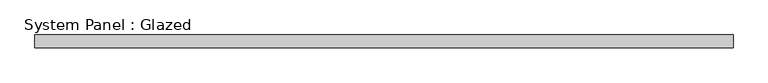
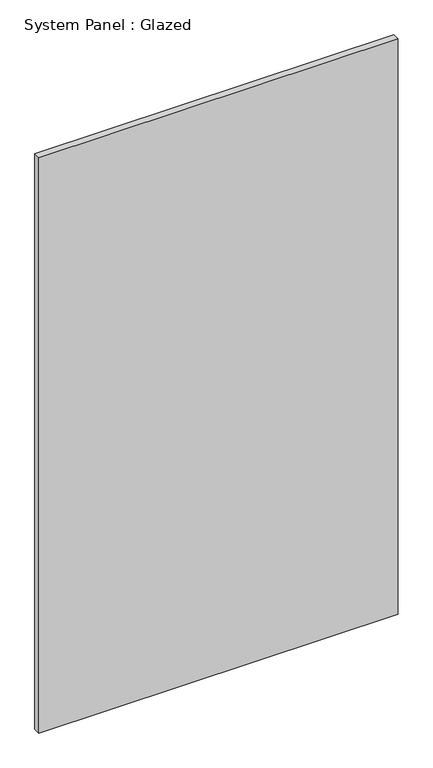
"""IFC4 building model written with IfcOpenShell, lengths in millimetres: plate geometry, System Panel : Glazed."""

from ifc_helpers import new_model, si_unit, origin, origin_with_axes, place, context, project, spatial, polyline, outline, extrude, source, transform, mapped, element, save


def system_panel_glazed_1dbb284f(model_context):
    return source(origin(), model_context, "Body", "SweptSolid", [
        extrude(outline(polyline([(692.15, 19.05), (-692.15, 19.05), (-692.15, 44.45), (692.15, 44.45), (692.15, 19.05)])), origin_with_axes(), (0.0, 0.0, 1.0), 2343.15),
    ])


if __name__ == "__main__":
    model = new_model("IFC4")
    model_context = context("Model", 3, world=origin())
    ifc_project = project(units=[si_unit("LENGTHUNIT", "METRE", prefix="MILLI")], contexts=[model_context])
    site = spatial("IfcSite", under=ifc_project)
    building = spatial("IfcBuilding", under=site)
    placement = place(None, origin())
    system_panel_glazed_shape = system_panel_glazed_1dbb284f(model_context)
    element("IfcPlate", 1, ObjectType="System Panel : Glazed", at=placement, inside=building, context=model_context, shape_type="MappedRepresentation", body=[
        mapped(system_panel_glazed_shape, transform((0.0, 0.0, 0.0), x_axis=(1.0, 0.0, 0.0), y_axis=(0.0, 1.0, 0.0), z_axis=(0.0, 0.0, 1.0))),
    ])
    save(model, "model.ifc")

# Revit data of these elements
# Type "System Panel : Glazed"
#   Construction Type Id = "GSP4R"
#   Analytic Construction = "1/8 in Pilkington single glazing"
#   Visual Light Transmittance = 0.9
#   Solar Heat Gain Coefficient = 0.86
#   Heat Transfer Coefficient (U) = 1.18115 BTU/(h·ft²·°F)
# Element 1 (IfcPlate, "System Panel : Glazed")
#   Materials on its faces: "Glass"
# Materials
#   "Glass": class "Glass", colour RGB 0 128 192, transparency 0.75, Description = "Soda Lime Glass", Cost = 0
